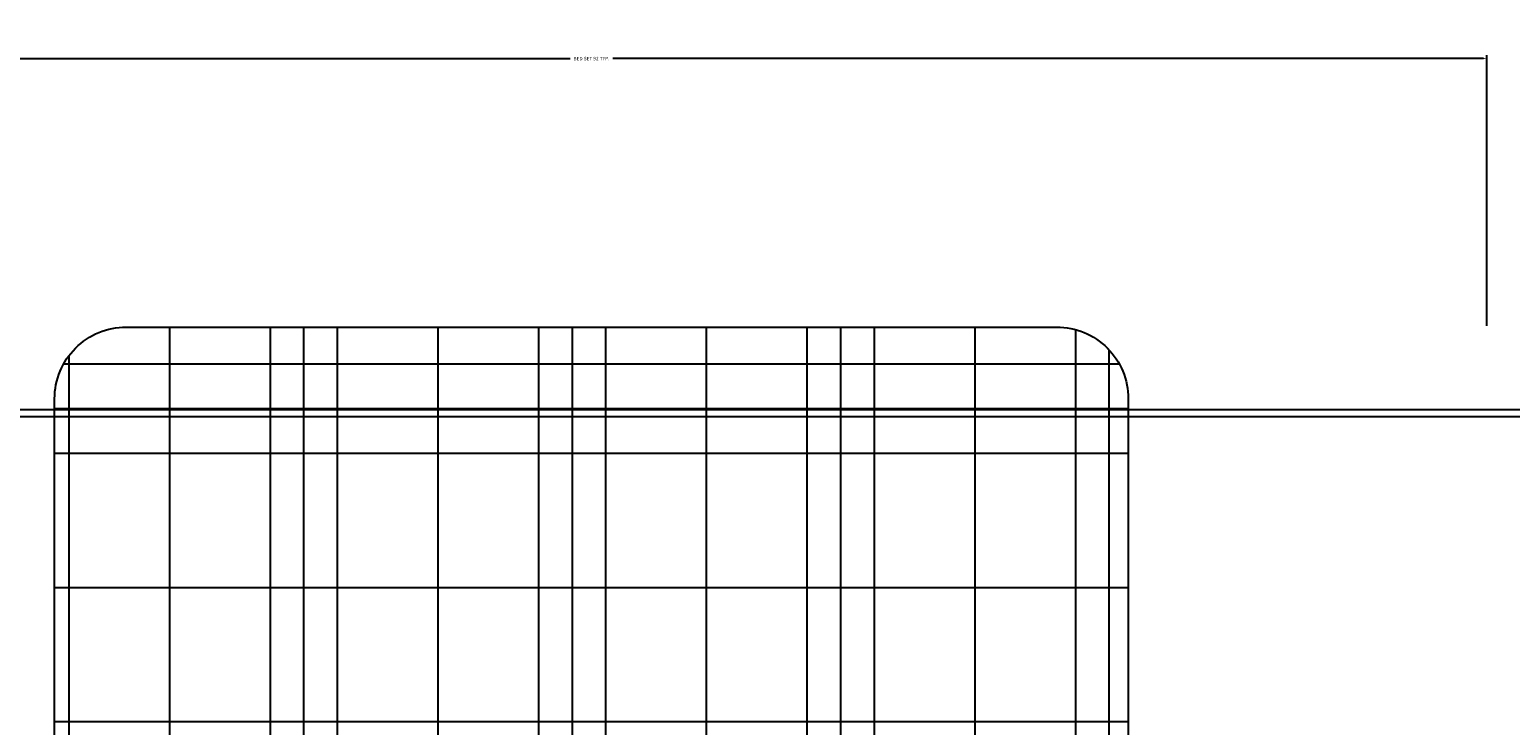
# Model space of a CAD drawing. Units: millimetres. Extents: x 2817 to 5038, y 1110 to 3565.
# Tile 16 of 21: x 2869 to 2946, y 1558 to 1593. Entities that reach past the tile are written whole.
import ezdxf

# ---------------------------------------------------------------- set-up
doc = ezdxf.new("R2010")
doc.units = ezdxf.units.MM
doc.layers.add('A-ANNO-DIMS', color=2, linetype='Continuous', lineweight=18)
doc.layers.add('FURNITURE', color=219, linetype='Continuous', lineweight=18)
doc.layers.add('BLOCK', color=6, linetype='Continuous')
doc.styles.get("Standard").update_dxf_attribs({"font": 'arial.ttf'})
doc.dimstyles.get("Standard").update_dxf_attribs({"dimtxt": 0.18, "dimasz": 0.18, "dimexe": 0.18, "dimexo": 0.0625, "dimgap": 0.09, "dimtad": 0, "dimtih": 1, "dimtoh": 1, "dimdec": 4, "dimzin": 0, "dimdsep": 46, "dimtxsty": 'Standard', "dimcen": 0.09, "dimadec": 0, "dimazin": 0, "dimtfac": 1, "dimtdec": 4, "dimtofl": 0, "dimtmove": 0, "dimatfit": 3, "dimfxl": 1, "dimtolj": 1, "dimtzin": 0, "dimarcsym": 0})

# ---------------------------------------------------------------- blocks, each defined once
blk = doc.blocks.new('*X7')
at = {"color": 0}
for p, q in [((276.598, 451.25), (280.51, 451.25)), ((275.455, 450.625), (280.51, 450.625)), ((274.411, 450), (280.51, 450)), ((265.51, 448.125), (267.634, 448.125)), ((271.723, 448.125), (280.51, 448.125)), ((265.51, 446.25), (268.465, 446.25)), ((269.519, 446.25), (280.51, 446.25)), ((265.51, 445.625), (268.531, 445.625)), ((268.866, 445.625), (280.51, 445.625)), ((265.51, 445), (280.51, 445)), ((265.51, 443.125), (280.51, 443.125)), ((265.51, 441.25), (280.51, 441.25)), ((265.51, 440.625), (280.51, 440.625)), ((265.634, 440), (280.386, 440))]:
    blk.add_line(p, q, dxfattribs=at)
blk = doc.blocks.new('*X8')
at = {"color": 0}
for p, q in [((280.312, 439.886), (280.312, 452.896)), ((278.906, 439.482), (278.906, 452.338)), ((277.5, 439.482), (277.5, 451.702)), ((277.031, 439.482), (277.031, 451.471)), ((276.562, 439.482), (276.562, 451.231)), ((275.156, 439.482), (275.156, 450.451)), ((273.75, 439.482), (273.75, 449.576)), ((265.781, 439.797), (265.781, 449.511)), ((266.25, 439.517), (266.25, 449.296)), ((273.281, 439.482), (273.281, 449.261)), ((272.812, 439.482), (272.812, 448.934)), ((267.656, 439.482), (267.656, 448.095)), ((271.406, 439.482), (271.406, 447.876)), ((270, 439.482), (270, 446.689)), ((269.531, 439.482), (269.531, 446.262)), ((269.062, 439.482), (269.062, 445.817))]:
    blk.add_line(p, q, dxfattribs=at)
blk = doc.blocks.new('A$C52E67D0D')
at = {"layer": 'BLOCK'}
blk.add_lwpolyline([(1901, 0), (601, 0, -0.414214), (501, 100), (501, 1700, -0.414214), (601, 1800), (1901, 1800, -0.414214), (2001, 1700), (2001, 100, -0.414214)], format="xyb", close=True, dxfattribs=at)
at = {"layer": 'BLOCK', "xscale": 100, "yscale": 100, "zscale": 100}
for name in ['*X8', '*X7']:
    blk.add_blockref(name, (-26050, -43948.2), dxfattribs=at)
blk = doc.blocks.new('*D18')
at = {"layer": 'A-ANNO-DIMS', "color": 0, "lineweight": -2, "transparency": 16777216}
for p, q in [((2852.329, 1578.101), (2852.329, 1592.019)), ((2852.509, 1591.839), (2897.232, 1591.839)), ((2944.149, 1591.839), (2899.426, 1591.839)), ((2944.329, 1578.101), (2944.329, 1592.019))]:
    blk.add_line(p, q, dxfattribs=at)
for points in [[(2852.509, 1591.869), (2852.509, 1591.809), (2852.329, 1591.839)], [(2944.149, 1591.869), (2944.149, 1591.809), (2944.329, 1591.839)]]:
    blk.add_solid(points, dxfattribs=at)
at = {"layer": 'Defpoints', "color": 0, "lineweight": -2, "transparency": 16777216}
for p in [(2852.329, 1591.839), (2852.329, 1578.039), (2944.329, 1578.039)]:
    blk.add_point(p, dxfattribs=at)
at = {"layer": 'A-ANNO-DIMS', "color": 0, "transparency": 16777216, "insert": (2898.329, 1591.839), "char_height": 0.18, "attachment_point": 5}
blk.add_mtext('\\A1;BED SET 92 TYP.', dxfattribs=at)
blk = doc.blocks.new('*D38')
at = {"layer": 'A-ANNO-DIMS', "color": 0, "lineweight": -2, "transparency": 16777216}
for p, q in [((3110.177, 1573.436), (2817.308, 1573.436)), ((2817.488, 1573.256), (2817.488, 1523.618)), ((2817.488, 1473.616), (2817.488, 1523.254)), ((3105.677, 1473.436), (2817.308, 1473.436))]:
    blk.add_line(p, q, dxfattribs=at)
for points in [[(2817.458, 1573.256), (2817.518, 1573.256), (2817.488, 1573.436)], [(2817.458, 1473.616), (2817.518, 1473.616), (2817.488, 1473.436)]]:
    blk.add_solid(points, dxfattribs=at)
at = {"layer": 'Defpoints', "color": 0, "lineweight": -2, "transparency": 16777216}
for p in [(2817.488, 1573.436), (3110.239, 1573.436), (3105.739, 1473.436)]:
    blk.add_point(p, dxfattribs=at)
at = {"layer": 'A-ANNO-DIMS', "color": 0, "transparency": 16777216, "insert": (2817.488, 1523.436), "char_height": 0.18, "attachment_point": 5}
blk.add_mtext('\\A1;100', dxfattribs=at)
blk = doc.blocks.new('*D39')
at = {"layer": 'A-ANNO-DIMS', "color": 0, "lineweight": -2, "transparency": 16777216}
for p, q in [((3105.677, 1605.436), (2817.308, 1605.436)), ((2817.488, 1605.256), (2817.488, 1589.618)), ((2817.488, 1573.616), (2817.488, 1589.254)), ((3110.177, 1573.436), (2817.308, 1573.436))]:
    blk.add_line(p, q, dxfattribs=at)
for points in [[(2817.458, 1605.256), (2817.518, 1605.256), (2817.488, 1605.436)], [(2817.458, 1573.616), (2817.518, 1573.616), (2817.488, 1573.436)]]:
    blk.add_solid(points, dxfattribs=at)
at = {"layer": 'Defpoints', "color": 0, "lineweight": -2, "transparency": 16777216}
for p in [(2817.488, 1605.436), (3105.739, 1605.436), (3110.239, 1573.436)]:
    blk.add_point(p, dxfattribs=at)
at = {"layer": 'A-ANNO-DIMS', "color": 0, "transparency": 16777216, "insert": (2817.488, 1589.436), "char_height": 0.18, "attachment_point": 5}
blk.add_mtext('\\A1;32', dxfattribs=at)
blk = doc.blocks.new('*D46')
at = {"layer": 'A-ANNO-DIMS', "color": 0, "lineweight": -2, "transparency": 16777216}
for p, q in [((3052.177, 1605.436), (2817.308, 1605.436)), ((2817.488, 1605.256), (2817.488, 1589.792)), ((2817.488, 1573.964), (2817.488, 1589.428)), ((3052.075, 1573.784), (2817.308, 1573.784))]:
    blk.add_line(p, q, dxfattribs=at)
for points in [[(2817.458, 1605.256), (2817.518, 1605.256), (2817.488, 1605.436)], [(2817.458, 1573.964), (2817.518, 1573.964), (2817.488, 1573.784)]]:
    blk.add_solid(points, dxfattribs=at)
at = {"layer": 'Defpoints', "color": 0, "lineweight": -2, "transparency": 16777216}
for p in [(2817.488, 1605.436), (3052.239, 1605.436), (3052.138, 1573.784)]:
    blk.add_point(p, dxfattribs=at)
at = {"layer": 'A-ANNO-DIMS', "color": 0, "transparency": 16777216, "insert": (2817.488, 1589.61), "char_height": 0.18, "attachment_point": 5}
blk.add_mtext('\\A1;31.65', dxfattribs=at)

msp = doc.modelspace()

# ---------------------------------------------------------------- block references
at = {"layer": 'FURNITURE', "xscale": 0.0367705835331598, "yscale": 0.0367705835331598, "zscale": 0.0367705835331598, "rotation": 180}
msp.add_blockref('A$C52E67D0D', (2944.3285, 1578.0385), dxfattribs=at)

# ---------------------------------------------------------------- dimensions: what is measured, and where the dimension line sits
at = {"layer": 'A-ANNO-DIMS'}
for base, p1, p2, override, picture, middle in [((2817.4881, 1605.4357), (3052.1378, 1573.7835), (3052.2393, 1605.4357), {"dimdec": 2, "dimlfac": 1, "dimrnd": 0, "dimzin": 0, "dimdsep": 46, "dimlunit": 2}, '*D46', (2817.4881, 1589.6096)), ((2817.4881, 1605.4357), (3110.2393, 1573.4357), (3105.7393, 1605.4357), {"dimdec": 0, "dimlfac": 1, "dimrnd": 0, "dimzin": 0, "dimdsep": 46, "dimlunit": 2}, '*D39', (2817.4881, 1589.4357)), ((2817.4881, 1573.4357), (3105.7393, 1473.4357), (3110.2393, 1573.4357), {"dimdec": 0, "dimlfac": 1, "dimrnd": 0, "dimzin": 0, "dimdsep": 46, "dimlunit": 2}, '*D38', (2817.4881, 1523.4357))]:
    dim = msp.add_linear_dim(base=base, p1=p1, p2=p2, angle=90, dimstyle='Standard', override=override, dxfattribs=at)
    dim.commit()
    dim.dimension.update_dxf_attribs({"geometry": picture, "text_midpoint": middle})
dim = msp.add_linear_dim(base=(2852.3285, 1591.8385), p1=(2944.3285, 1578.0385), p2=(2852.3285, 1578.0385), angle=180, text='BED SET <> TYP.', dimstyle='Standard', override={"dimdec": 0, "dimlfac": 1, "dimrnd": 0, "dimzin": 0, "dimdsep": 46, "dimlunit": 2}, dxfattribs=at)
dim.commit()
dim.dimension.update_dxf_attribs({"geometry": '*D18', "text_midpoint": (2898.3285, 1591.8385)})

doc.saveas('drawing.dxf')
